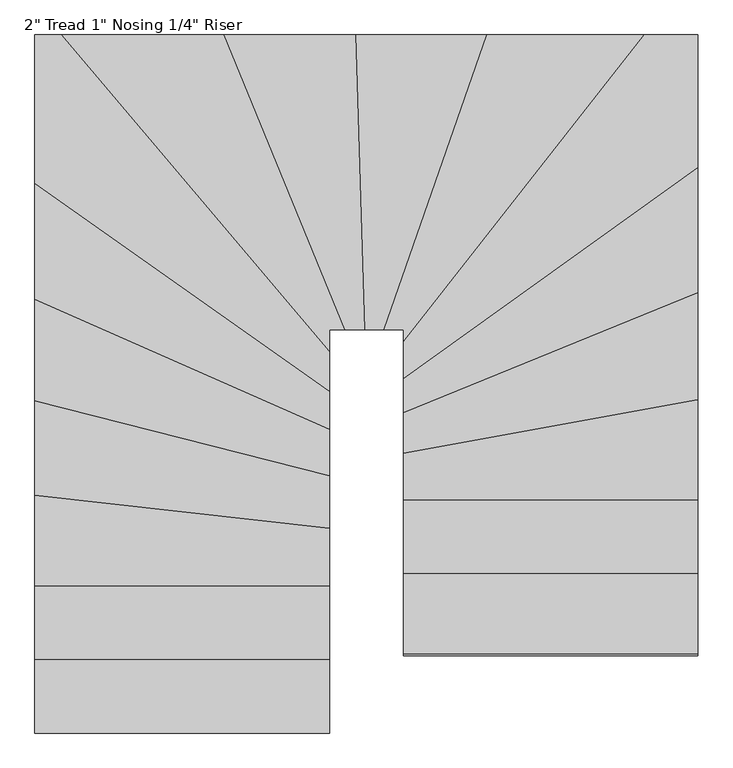
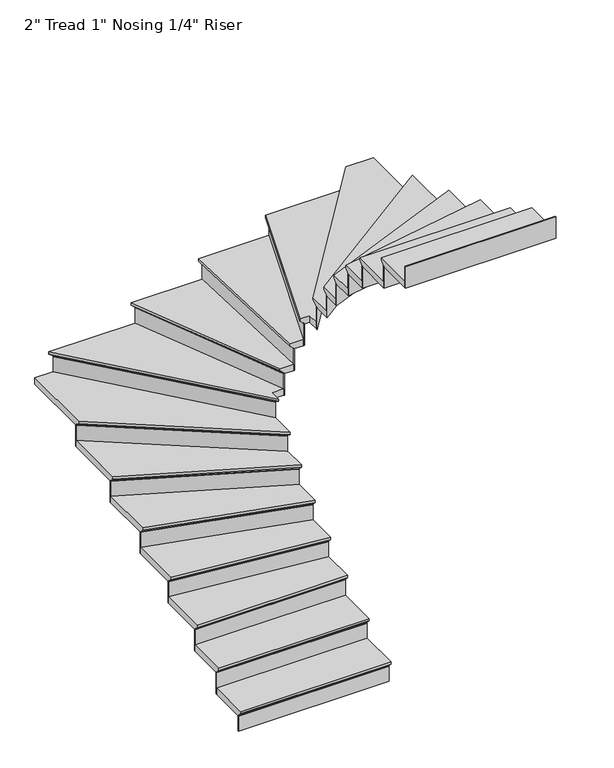
"""IFC4 building model written with IfcOpenShell, lengths in millimetres: stair flight geometry."""

from ifc_helpers import new_model, si_unit, origin, place, context, project, spatial, faceted_brep, source, transform, mapped, element, save


def stair_flight_2fadb1b5(model_context):
    return source(origin(), model_context, "Body", "Brep", [
        faceted_brep([(-7924.9808972, 1205.8606436, 150.2833333), (-7924.9808972, 1205.8606436, 169.3333333), (-9042.5808972, 1205.8606436, 169.3333333), (-9042.5808972, 1205.8606436, 150.2833333), (-7924.9808972, 1231.2606436, 124.8833333), (-9042.5808972, 1231.2606436, 124.8833333), (-7924.9808972, 1510.6606436, 169.3333333), (-9042.5808972, 1510.6606436, 169.3333333), (-9042.5808972, 1231.2606436, 118.5333333), (-9042.5808972, 1510.6606436, 118.5333333), (-7924.9808972, 1510.6606436, 118.5333333), (-7924.9808972, 1231.2606436, 118.5333333)], [[[0, 1, 2, 3]], [[4, 0, 3, 5]], [[2, 1, 6, 7]], [[8, 9, 10, 11]], [[2, 7, 9, 8, 5, 3]], [[8, 11, 4, 5]], [[6, 1, 0, 4, 11, 10]], [[7, 6, 10, 9]]]),
        faceted_brep([(-7924.9808972, 1231.2606436, 118.5333333), (-7924.9808972, 1231.2606436, 0.0), (-7924.9808972, 1237.6106436, 0.0), (-7924.9808972, 1237.6106436, 118.5333333), (-9042.5808972, 1231.2606436, 118.5333333), (-9042.5808972, 1237.6106436, 118.5333333), (-9042.5808972, 1237.6106436, 0.0), (-9042.5808972, 1231.2606436, 0.0)], [[[0, 1, 2, 3]], [[4, 5, 6, 7]], [[1, 0, 4, 7]], [[2, 1, 7, 6]], [[3, 2, 6, 5]], [[0, 3, 5, 4]]]),
        faceted_brep([(-7924.9808972, 1510.6606436, 287.8666667), (-7924.9808972, 1510.6606436, 118.5333333), (-7924.9808972, 1517.0106436, 118.5333333), (-7924.9808972, 1517.0106436, 287.8666667), (-9042.5808972, 1510.6606436, 287.8666667), (-9042.5808972, 1517.0106436, 287.8666667), (-9042.5808972, 1517.0106436, 118.5333333), (-9042.5808972, 1510.6606436, 118.5333333)], [[[0, 1, 2, 3]], [[4, 5, 6, 7]], [[1, 0, 4, 7]], [[2, 1, 7, 6]], [[3, 2, 6, 5]], [[0, 3, 5, 4]]]),
        faceted_brep([(-9042.5808972, 1485.2606436, 338.6666667), (-7924.9808972, 1485.2606436, 338.6666667), (-7924.9808972, 1790.0606436, 338.6666667), (-9042.5808972, 1790.0606436, 338.6666667), (-9042.5808972, 1510.6606436, 287.8666667), (-9042.5808972, 1790.0606436, 287.8666667), (-7924.9808972, 1790.0606436, 287.8666667), (-7924.9808972, 1510.6606436, 287.8666667), (-9042.5808972, 1510.6606436, 294.2166667), (-9042.5808972, 1485.2606436, 319.6166667), (-7924.9808972, 1510.6606436, 294.2166667), (-7924.9808972, 1485.2606436, 319.6166667)], [[[0, 1, 2, 3]], [[4, 5, 6, 7]], [[0, 3, 5, 4, 8, 9]], [[4, 7, 10, 8]], [[2, 1, 11, 10, 7, 6]], [[3, 2, 6, 5]], [[11, 1, 0, 9]], [[10, 11, 9, 8]]]),
        faceted_brep([(-7924.9808972, 1790.0606436, 457.2), (-7924.9808972, 1790.0606436, 287.8666667), (-7924.9808972, 1796.4106436, 287.8666667), (-7924.9808972, 1796.4106436, 457.2), (-9042.5808972, 1790.0606436, 457.2), (-9042.5808972, 1796.4106436, 457.2), (-9042.5808972, 1796.4106436, 287.8666667), (-9042.5808972, 1790.0606436, 287.8666667)], [[[0, 1, 2, 3]], [[4, 5, 6, 7]], [[1, 0, 4, 7]], [[2, 1, 7, 6]], [[3, 2, 6, 5]], [[0, 3, 5, 4]]]),
        faceted_brep([(-9042.5808972, 1764.6606436, 508.0), (-7924.9808972, 1764.6606436, 508.0), (-7924.9808972, 2006.9009022, 508.0), (-9042.5808972, 2132.3393631, 508.0), (-9042.5808972, 1790.0606436, 457.2), (-9042.5808972, 2132.3393631, 457.2), (-7924.9808972, 2006.9009022, 457.2), (-7924.9808972, 1790.0606436, 457.2), (-9042.5808972, 1790.0606436, 463.55), (-9042.5808972, 1764.6606436, 488.95), (-7924.9808972, 1790.0606436, 463.55), (-7924.9808972, 1764.6606436, 488.95)], [[[0, 1, 2, 3]], [[4, 5, 6, 7]], [[0, 3, 5, 4, 8, 9]], [[4, 7, 10, 8]], [[2, 1, 11, 10, 7, 6]], [[3, 2, 6, 5]], [[11, 1, 0, 9]], [[10, 11, 9, 8]]]),
        faceted_brep([(-7924.9808972, 2006.9009022, 626.5333333), (-7924.9808972, 2006.9009022, 457.2), (-7924.9808972, 2013.2907745, 457.2), (-7924.9808972, 2013.2907745, 626.5333333), (-9042.5808972, 2132.3393631, 626.5333333), (-9042.5808972, 2138.7292354, 626.5333333), (-9042.5808972, 2138.7292354, 457.2), (-9042.5808972, 2132.3393631, 457.2)], [[[0, 1, 2, 3]], [[4, 5, 6, 7]], [[1, 0, 4, 7]], [[2, 1, 7, 6]], [[3, 2, 6, 5]], [[0, 3, 5, 4]]]),
        faceted_brep([(-9042.5808972, 2106.779874, 677.3333333), (-7924.9808972, 1981.3414131, 677.3333333), (-7924.9808972, 2207.3909228, 677.3333333), (-9042.5808972, 2491.9511882, 677.3333333), (-9042.5808972, 2132.3393631, 626.5333333), (-9042.5808972, 2491.9511882, 626.5333333), (-7924.9808972, 2207.3909228, 626.5333333), (-7924.9808972, 2006.9009022, 626.5333333), (-9042.5808972, 2132.3393631, 632.8833333), (-9042.5808972, 2106.779874, 658.2833333), (-7924.9808972, 2006.9009022, 632.8833333), (-7924.9808972, 1981.3414131, 658.2833333)], [[[0, 1, 2, 3]], [[4, 5, 6, 7]], [[0, 3, 5, 4, 8, 9]], [[4, 7, 10, 8]], [[2, 1, 11, 10, 7, 6]], [[3, 2, 6, 5]], [[11, 1, 0, 9]], [[10, 11, 9, 8]]]),
        faceted_brep([(-7924.9808972, 2207.3909228, 795.8666667), (-7924.9808972, 2207.3909228, 626.5333333), (-7924.9808972, 2213.9435258, 626.5333333), (-7924.9808972, 2213.9435258, 795.8666667), (-9042.5808972, 2491.9511882, 795.8666667), (-9042.5808972, 2498.5037912, 795.8666667), (-9042.5808972, 2498.5037912, 626.5333333), (-9042.5808972, 2491.9511882, 626.5333333)], [[[0, 1, 2, 3]], [[4, 5, 6, 7]], [[1, 0, 4, 7]], [[2, 1, 7, 6]], [[3, 2, 6, 5]], [[0, 3, 5, 4]]]),
        faceted_brep([(-9042.5808972, 2465.7407763, 846.6666667), (-7924.9808972, 2181.1805109, 846.6666667), (-7924.9808972, 2384.1041471, 846.6666667), (-9042.5808972, 2877.1408478, 846.6666667), (-9042.5808972, 2491.9511882, 795.8666667), (-9042.5808972, 2877.1408478, 795.8666667), (-7924.9808972, 2384.1041471, 795.8666667), (-7924.9808972, 2207.3909228, 795.8666667), (-9042.5808972, 2491.9511882, 802.2166667), (-9042.5808972, 2465.7407763, 827.6166667), (-7924.9808972, 2207.3909228, 802.2166667), (-7924.9808972, 2181.1805109, 827.6166667)], [[[0, 1, 2, 3]], [[4, 5, 6, 7]], [[0, 3, 5, 4, 8, 9]], [[4, 7, 10, 8]], [[2, 1, 11, 10, 7, 6]], [[3, 2, 6, 5]], [[11, 1, 0, 9]], [[10, 11, 9, 8]]]),
        faceted_brep([(-7924.9808972, 2384.1041471, 965.2), (-7924.9808972, 2384.1041471, 795.8666667), (-7924.9808972, 2391.0446106, 795.8666667), (-7924.9808972, 2391.0446106, 965.2), (-9042.5808972, 2877.1408478, 965.2), (-9042.5808972, 2884.0813113, 965.2), (-9042.5808972, 2884.0813113, 795.8666667), (-9042.5808972, 2877.1408478, 795.8666667)], [[[0, 1, 2, 3]], [[4, 5, 6, 7]], [[1, 0, 4, 7]], [[2, 1, 7, 6]], [[3, 2, 6, 5]], [[0, 3, 5, 4]]]),
        faceted_brep([(-9042.5808972, 2849.3789939, 1016.0), (-7924.9808972, 2356.3422932, 1016.0), (-7924.9808972, 2533.0028357, 1016.0), (-9042.5808972, 3320.3326574, 1016.0), (-9042.5808972, 2877.1408478, 965.2), (-9042.5808972, 3320.3326574, 965.2), (-7924.9808972, 2533.0028357, 965.2), (-7924.9808972, 2384.1041471, 965.2), (-9042.5808972, 2877.1408478, 971.55), (-9042.5808972, 2849.3789939, 996.95), (-7924.9808972, 2384.1041471, 971.55), (-7924.9808972, 2356.3422932, 996.95)], [[[0, 1, 2, 3]], [[4, 5, 6, 7]], [[0, 3, 5, 4, 8, 9]], [[4, 7, 10, 8]], [[2, 1, 11, 10, 7, 6]], [[3, 2, 6, 5]], [[11, 1, 0, 9]], [[10, 11, 9, 8]]]),
        faceted_brep([(-7924.9808972, 2533.0028357, 1134.5333333), (-7924.9808972, 2533.0028357, 965.2), (-7924.9808972, 2540.770357, 965.2), (-7924.9808972, 2540.770357, 1134.5333333), (-9042.5808972, 3320.3326574, 1134.5333333), (-9042.5808972, 3328.1001788, 1134.5333333), (-9042.5808972, 3328.1001788, 965.2), (-9042.5808972, 3320.3326574, 965.2)], [[[0, 1, 2, 3]], [[4, 5, 6, 7]], [[1, 0, 4, 7]], [[2, 1, 7, 6]], [[3, 2, 6, 5]], [[0, 3, 5, 4]]]),
        faceted_brep([(-8907.7976269, 3851.1923354, 1185.3333333), (-9042.5808972, 3851.1923354, 1185.3333333), (-9042.5808972, 3289.2625719, 1185.3333333), (-7924.9808972, 2501.9327502, 1185.3333333), (-7924.9808972, 2691.3009895, 1185.3333333), (-9042.5808972, 3851.1923354, 1134.5333333), (-8907.7976269, 3851.1923354, 1134.5333333), (-7924.9808972, 2691.3009895, 1134.5333333), (-7924.9808972, 2533.0028357, 1134.5333333), (-9042.5808972, 3320.3326574, 1134.5333333), (-9042.5808972, 3320.3326574, 1140.8833333), (-9042.5808972, 3289.2625719, 1166.2833333), (-7924.9808972, 2533.0028357, 1140.8833333), (-7924.9808972, 2501.9327502, 1166.2833333)], [[[0, 1, 2, 3, 4]], [[5, 6, 7, 8, 9]], [[1, 0, 6, 5]], [[2, 1, 5, 9, 10, 11]], [[9, 8, 12, 10]], [[4, 3, 13, 12, 8, 7]], [[0, 4, 7, 6]], [[13, 3, 2, 11]], [[12, 13, 11, 10]]]),
        faceted_brep([(-7924.9808972, 2691.3009895, 1303.8666667), (-7924.9808972, 2691.3009895, 1134.5333333), (-7924.9808972, 2701.1236052, 1134.5333333), (-7924.9808972, 2701.1236052, 1303.8666667), (-8907.7976269, 3851.1923354, 1303.8666667), (-8899.4745792, 3851.1923354, 1303.8666667), (-8899.4745792, 3851.1923354, 1134.5333333), (-8907.7976269, 3851.1923354, 1134.5333333)], [[[0, 1, 2, 3]], [[4, 5, 6, 7]], [[1, 0, 4, 7]], [[2, 1, 7, 6]], [[3, 2, 6, 5]], [[0, 3, 5, 4]]]),
        faceted_brep([(-8941.0898177, 3851.1923354, 1354.6666667), (-7924.9808972, 2652.0105269, 1354.6666667), (-7924.9808972, 2733.5923354, 1354.6666667), (-7838.5095187, 2733.5923354, 1354.6666667), (-8297.8208023, 3851.1923354, 1354.6666667), (-8907.7976269, 3851.1923354, 1303.8666667), (-8297.8208023, 3851.1923354, 1303.8666667), (-7838.5095187, 2733.5923354, 1303.8666667), (-7924.9808972, 2733.5923354, 1303.8666667), (-7924.9808972, 2691.3009895, 1303.8666667), (-8907.7976269, 3851.1923354, 1310.2166667), (-8941.0898177, 3851.1923354, 1335.6166667), (-7924.9808972, 2691.3009895, 1310.2166667), (-7924.9808972, 2652.0105269, 1335.6166667)], [[[0, 1, 2, 3, 4]], [[5, 6, 7, 8, 9]], [[0, 4, 6, 5, 10, 11]], [[5, 9, 12, 10]], [[3, 2, 8, 7]], [[4, 3, 7, 6]], [[13, 1, 0, 11]], [[12, 13, 11, 10]], [[2, 1, 13, 12, 9, 8]]]),
        faceted_brep([(-7838.5095187, 2733.5923354, 1473.2), (-7838.5095187, 2733.5923354, 1303.8666667), (-7831.6441596, 2733.5923354, 1303.8666667), (-7831.6441596, 2733.5923354, 1473.2), (-8297.8208023, 3851.1923354, 1473.2), (-8290.9554433, 3851.1923354, 1473.2), (-8290.9554433, 3851.1923354, 1303.8666667), (-8297.8208023, 3851.1923354, 1303.8666667)], [[[0, 1, 2, 3]], [[4, 5, 6, 7]], [[1, 0, 4, 7]], [[2, 1, 7, 6]], [[3, 2, 6, 5]], [[0, 3, 5, 4]]]),
        faceted_brep([(-8325.2822386, 3851.1923354, 1524.0), (-7865.970955, 2733.5923354, 1524.0), (-7765.6019906, 2733.5923354, 1524.0), (-7798.581504, 3851.1923354, 1524.0), (-8297.8208023, 3851.1923354, 1473.2), (-7798.581504, 3851.1923354, 1473.2), (-7765.6019906, 2733.5923354, 1473.2), (-7838.5095187, 2733.5923354, 1473.2), (-8297.8208023, 3851.1923354, 1479.55), (-8325.2822386, 3851.1923354, 1504.95), (-7838.5095187, 2733.5923354, 1479.55), (-7865.970955, 2733.5923354, 1504.95)], [[[0, 1, 2, 3]], [[4, 5, 6, 7]], [[0, 3, 5, 4, 8, 9]], [[4, 7, 10, 8]], [[2, 1, 11, 10, 7, 6]], [[3, 2, 6, 5]], [[11, 1, 0, 9]], [[10, 11, 9, 8]]]),
        faceted_brep([(-7765.6019906, 2733.5923354, 1642.5333333), (-7765.6019906, 2733.5923354, 1473.2), (-7759.2492264, 2733.5923354, 1473.2), (-7759.2492264, 2733.5923354, 1642.5333333), (-7798.581504, 3851.1923354, 1642.5333333), (-7792.2287398, 3851.1923354, 1642.5333333), (-7792.2287398, 3851.1923354, 1473.2), (-7798.581504, 3851.1923354, 1473.2)], [[[0, 1, 2, 3]], [[4, 5, 6, 7]], [[1, 0, 4, 7]], [[2, 1, 7, 6]], [[3, 2, 6, 5]], [[0, 3, 5, 4]]]),
        faceted_brep([(-7823.9925607, 3851.1923354, 1693.3333333), (-7791.0130473, 2733.5923354, 1693.3333333), (-7692.111373, 2733.5923354, 1693.3333333), (-7302.1708713, 3851.1923354, 1693.3333333), (-7798.581504, 3851.1923354, 1642.5333333), (-7302.1708713, 3851.1923354, 1642.5333333), (-7692.111373, 2733.5923354, 1642.5333333), (-7765.6019906, 2733.5923354, 1642.5333333), (-7798.581504, 3851.1923354, 1648.8833333), (-7823.9925607, 3851.1923354, 1674.2833333), (-7765.6019906, 2733.5923354, 1648.8833333), (-7791.0130473, 2733.5923354, 1674.2833333)], [[[0, 1, 2, 3]], [[4, 5, 6, 7]], [[0, 3, 5, 4, 8, 9]], [[4, 7, 10, 8]], [[2, 1, 11, 10, 7, 6]], [[3, 2, 6, 5]], [[11, 1, 0, 9]], [[10, 11, 9, 8]]]),
        faceted_brep([(-7692.111373, 2733.5923354, 1811.8666667), (-7692.111373, 2733.5923354, 1642.5333333), (-7685.3859544, 2733.5923354, 1642.5333333), (-7685.3859544, 2733.5923354, 1811.8666667), (-7302.1708713, 3851.1923354, 1811.8666667), (-7295.4454527, 3851.1923354, 1811.8666667), (-7295.4454527, 3851.1923354, 1642.5333333), (-7302.1708713, 3851.1923354, 1642.5333333)], [[[0, 1, 2, 3]], [[4, 5, 6, 7]], [[1, 0, 4, 7]], [[2, 1, 7, 6]], [[3, 2, 6, 5]], [[0, 3, 5, 4]]]),
        faceted_brep([(-7329.0725456, 3851.1923354, 1862.6666667), (-7719.0130473, 2733.5923354, 1862.6666667), (-7645.5808972, 2733.5923354, 1862.6666667), (-7645.5808972, 2646.5119616, 1862.6666667), (-6699.3018022, 3851.1923354, 1862.6666667), (-7302.1708713, 3851.1923354, 1811.8666667), (-6699.3018022, 3851.1923354, 1811.8666667), (-7645.5808972, 2646.5119616, 1811.8666667), (-7645.5808972, 2733.5923354, 1811.8666667), (-7692.111373, 2733.5923354, 1811.8666667), (-7302.1708713, 3851.1923354, 1818.2166667), (-7329.0725456, 3851.1923354, 1843.6166667), (-7692.111373, 2733.5923354, 1818.2166667), (-7719.0130473, 2733.5923354, 1843.6166667)], [[[0, 1, 2, 3, 4]], [[5, 6, 7, 8, 9]], [[0, 4, 6, 5, 10, 11]], [[5, 9, 12, 10]], [[2, 1, 13, 12, 9, 8]], [[4, 3, 7, 6]], [[13, 1, 0, 11]], [[12, 13, 11, 10]], [[3, 2, 8, 7]]]),
        faceted_brep([(-7645.5808972, 2646.5119616, 1981.2), (-7645.5808972, 2646.5119616, 1811.8666667), (-7645.5808972, 2636.2321971, 1811.8666667), (-7645.5808972, 2636.2321971, 1981.2), (-6699.3018022, 3851.1923354, 1981.2), (-6691.2270245, 3851.1923354, 1981.2), (-6691.2270245, 3851.1923354, 1811.8666667), (-6699.3018022, 3851.1923354, 1811.8666667)], [[[0, 1, 2, 3]], [[4, 5, 6, 7]], [[1, 0, 4, 7]], [[2, 1, 7, 6]], [[3, 2, 6, 5]], [[0, 3, 5, 4]]]),
        faceted_brep([(-6527.9808972, 3317.4403684, 2032.0), (-6527.9808972, 3851.1923354, 2032.0), (-6731.6009132, 3851.1923354, 2032.0), (-7645.5808972, 2687.6310198, 2032.0), (-7645.5808972, 2517.3671111, 2032.0), (-6527.9808972, 3851.1923354, 1981.2), (-6527.9808972, 3317.4403684, 1981.2), (-7645.5808972, 2517.3671111, 1981.2), (-7645.5808972, 2646.5119616, 1981.2), (-6699.3018022, 3851.1923354, 1981.2), (-7645.5808972, 2646.5119616, 1987.55), (-6699.3018022, 3851.1923354, 1987.55), (-7645.5808972, 2687.6310198, 2012.95), (-6731.6009132, 3851.1923354, 2012.95)], [[[0, 1, 2, 3, 4]], [[5, 6, 7, 8, 9]], [[1, 0, 6, 5]], [[9, 8, 10, 11]], [[4, 3, 12, 10, 8, 7]], [[0, 4, 7, 6]], [[12, 3, 2, 13]], [[10, 12, 13, 11]], [[2, 1, 5, 9, 11, 13]]]),
        faceted_brep([(-7645.5808972, 2517.3671111, 2150.5333333), (-7645.5808972, 2517.3671111, 1981.2), (-7645.5808972, 2509.5576655, 1981.2), (-7645.5808972, 2509.5576655, 2150.5333333), (-6527.9808972, 3317.4403684, 2150.5333333), (-6527.9808972, 3309.6309228, 2150.5333333), (-6527.9808972, 3309.6309228, 1981.2), (-6527.9808972, 3317.4403684, 1981.2)], [[[0, 1, 2, 3]], [[4, 5, 6, 7]], [[1, 0, 4, 7]], [[2, 1, 7, 6]], [[3, 2, 6, 5]], [[0, 3, 5, 4]]]),
        faceted_brep([(-6527.9808972, 3348.678151, 2201.3333333), (-7645.5808972, 2548.6048936, 2201.3333333), (-7645.5808972, 2392.4773927, 2201.3333333), (-6527.9808972, 2847.0609144, 2201.3333333), (-6527.9808972, 3317.4403684, 2150.5333333), (-6527.9808972, 2847.0609144, 2150.5333333), (-7645.5808972, 2392.4773927, 2150.5333333), (-7645.5808972, 2517.3671111, 2150.5333333), (-6527.9808972, 3317.4403684, 2156.8833333), (-6527.9808972, 3348.678151, 2182.2833333), (-7645.5808972, 2517.3671111, 2156.8833333), (-7645.5808972, 2548.6048936, 2182.2833333)], [[[0, 1, 2, 3]], [[4, 5, 6, 7]], [[0, 3, 5, 4, 8, 9]], [[4, 7, 10, 8]], [[2, 1, 11, 10, 7, 6]], [[3, 2, 6, 5]], [[11, 1, 0, 9]], [[10, 11, 9, 8]]]),
        faceted_brep([(-7645.5808972, 2392.4773927, 2319.8666667), (-7645.5808972, 2392.4773927, 2150.5333333), (-7645.5808972, 2385.6221998, 2150.5333333), (-7645.5808972, 2385.6221998, 2319.8666667), (-6527.9808972, 2847.0609144, 2319.8666667), (-6527.9808972, 2840.2057215, 2319.8666667), (-6527.9808972, 2840.2057215, 2150.5333333), (-6527.9808972, 2847.0609144, 2150.5333333)], [[[0, 1, 2, 3]], [[4, 5, 6, 7]], [[1, 0, 4, 7]], [[2, 1, 7, 6]], [[3, 2, 6, 5]], [[0, 3, 5, 4]]]),
        faceted_brep([(-6527.9808972, 2874.4816863, 2370.6666667), (-7645.5808972, 2419.8981646, 2370.6666667), (-7645.5808972, 2240.9879192, 2370.6666667), (-6527.9808972, 2442.9689719, 2370.6666667), (-6527.9808972, 2847.0609144, 2319.8666667), (-6527.9808972, 2442.9689719, 2319.8666667), (-7645.5808972, 2240.9879192, 2319.8666667), (-7645.5808972, 2392.4773927, 2319.8666667), (-6527.9808972, 2847.0609144, 2326.2166667), (-6527.9808972, 2874.4816863, 2351.6166667), (-7645.5808972, 2392.4773927, 2326.2166667), (-7645.5808972, 2419.8981646, 2351.6166667)], [[[0, 1, 2, 3]], [[4, 5, 6, 7]], [[0, 3, 5, 4, 8, 9]], [[4, 7, 10, 8]], [[2, 1, 11, 10, 7, 6]], [[3, 2, 6, 5]], [[11, 1, 0, 9]], [[10, 11, 9, 8]]]),
        faceted_brep([(-7645.5808972, 2240.9879192, 2489.2), (-7645.5808972, 2240.9879192, 2319.8666667), (-7645.5808972, 2234.5350493, 2319.8666667), (-7645.5808972, 2234.5350493, 2489.2), (-6527.9808972, 2442.9689719, 2489.2), (-6527.9808972, 2436.5161019, 2489.2), (-6527.9808972, 2436.5161019, 2319.8666667), (-6527.9808972, 2442.9689719, 2319.8666667)], [[[0, 1, 2, 3]], [[4, 5, 6, 7]], [[1, 0, 4, 7]], [[2, 1, 7, 6]], [[3, 2, 6, 5]], [[0, 3, 5, 4]]]),
        faceted_brep([(-6527.9808972, 2468.7804518, 2540.0), (-7645.5808972, 2266.7993991, 2540.0), (-7645.5808972, 2062.9899254, 2540.0), (-6527.9808972, 2062.9899254, 2540.0), (-6527.9808972, 2442.9689719, 2489.2), (-6527.9808972, 2062.9899254, 2489.2), (-7645.5808972, 2062.9899254, 2489.2), (-7645.5808972, 2240.9879192, 2489.2), (-6527.9808972, 2442.9689719, 2495.55), (-6527.9808972, 2468.7804518, 2520.95), (-7645.5808972, 2240.9879192, 2495.55), (-7645.5808972, 2266.7993991, 2520.95)], [[[0, 1, 2, 3]], [[4, 5, 6, 7]], [[0, 3, 5, 4, 8, 9]], [[4, 7, 10, 8]], [[2, 1, 11, 10, 7, 6]], [[3, 2, 6, 5]], [[11, 1, 0, 9]], [[10, 11, 9, 8]]]),
        faceted_brep([(-7645.5808972, 2062.9899254, 2658.5333333), (-7645.5808972, 2062.9899254, 2489.2), (-7645.5808972, 2056.6399254, 2489.2), (-7645.5808972, 2056.6399254, 2658.5333333), (-6527.9808972, 2062.9899254, 2658.5333333), (-6527.9808972, 2056.6399254, 2658.5333333), (-6527.9808972, 2056.6399254, 2489.2), (-6527.9808972, 2062.9899254, 2489.2)], [[[0, 1, 2, 3]], [[4, 5, 6, 7]], [[1, 0, 4, 7]], [[2, 1, 7, 6]], [[3, 2, 6, 5]], [[0, 3, 5, 4]]]),
        faceted_brep([(-6527.9808972, 2088.3899254, 2709.3333333), (-7645.5808972, 2088.3899254, 2709.3333333), (-7645.5808972, 1783.5899254, 2709.3333333), (-6527.9808972, 1783.5899254, 2709.3333333), (-6527.9808972, 2062.9899254, 2658.5333333), (-6527.9808972, 1783.5899254, 2658.5333333), (-7645.5808972, 1783.5899254, 2658.5333333), (-7645.5808972, 2062.9899254, 2658.5333333), (-6527.9808972, 2062.9899254, 2664.8833333), (-6527.9808972, 2088.3899254, 2690.2833333), (-7645.5808972, 2062.9899254, 2664.8833333), (-7645.5808972, 2088.3899254, 2690.2833333)], [[[0, 1, 2, 3]], [[4, 5, 6, 7]], [[0, 3, 5, 4, 8, 9]], [[4, 7, 10, 8]], [[2, 1, 11, 10, 7, 6]], [[3, 2, 6, 5]], [[11, 1, 0, 9]], [[10, 11, 9, 8]]]),
        faceted_brep([(-7645.5808972, 1783.5899254, 2827.8666667), (-7645.5808972, 1783.5899254, 2658.5333333), (-7645.5808972, 1777.2399254, 2658.5333333), (-7645.5808972, 1777.2399254, 2827.8666667), (-6527.9808972, 1783.5899254, 2827.8666667), (-6527.9808972, 1777.2399254, 2827.8666667), (-6527.9808972, 1777.2399254, 2658.5333333), (-6527.9808972, 1783.5899254, 2658.5333333)], [[[0, 1, 2, 3]], [[4, 5, 6, 7]], [[1, 0, 4, 7]], [[2, 1, 7, 6]], [[3, 2, 6, 5]], [[0, 3, 5, 4]]]),
        faceted_brep([(-7645.5808972, 1504.1899254, 2997.2), (-7645.5808972, 1504.1899254, 2827.8666667), (-7645.5808972, 1497.8399254, 2827.8666667), (-7645.5808972, 1497.8399254, 2997.2), (-6527.9808972, 1504.1899254, 2997.2), (-6527.9808972, 1497.8399254, 2997.2), (-6527.9808972, 1497.8399254, 2827.8666667), (-6527.9808972, 1504.1899254, 2827.8666667)], [[[0, 1, 2, 3]], [[4, 5, 6, 7]], [[1, 0, 4, 7]], [[2, 1, 7, 6]], [[3, 2, 6, 5]], [[0, 3, 5, 4]]]),
        faceted_brep([(-6527.9808972, 1808.9899254, 2878.6666667), (-7645.5808972, 1808.9899254, 2878.6666667), (-7645.5808972, 1504.1899254, 2878.6666667), (-6527.9808972, 1504.1899254, 2878.6666667), (-6527.9808972, 1783.5899254, 2827.8666667), (-6527.9808972, 1504.1899254, 2827.8666667), (-7645.5808972, 1504.1899254, 2827.8666667), (-7645.5808972, 1783.5899254, 2827.8666667), (-6527.9808972, 1783.5899254, 2834.2166667), (-6527.9808972, 1808.9899254, 2859.6166667), (-7645.5808972, 1783.5899254, 2834.2166667), (-7645.5808972, 1808.9899254, 2859.6166667)], [[[0, 1, 2, 3]], [[4, 5, 6, 7]], [[0, 3, 5, 4, 8, 9]], [[4, 7, 10, 8]], [[2, 1, 11, 10, 7, 6]], [[3, 2, 6, 5]], [[11, 1, 0, 9]], [[10, 11, 9, 8]]]),
    ])


if __name__ == "__main__":
    model = new_model("IFC4")
    model_context = context("Model", 3, world=origin())
    ifc_project = project(units=[si_unit("LENGTHUNIT", "METRE", prefix="MILLI")], contexts=[model_context])
    site = spatial("IfcSite", under=ifc_project)
    building = spatial("IfcBuilding", under=site)
    placement = place(None, origin())
    stair_flight_shape = stair_flight_2fadb1b5(model_context)
    element("IfcStairFlight", 1, ObjectType="2\" Tread 1\" Nosing 1/4\" Riser", at=placement, inside=building, context=model_context, shape_type="MappedRepresentation", body=[
        mapped(stair_flight_shape, transform((0.0, 0.0, 0.0), x_axis=(1.0, 0.0, 0.0), y_axis=(0.0, 1.0, 0.0), z_axis=(0.0, 0.0, 1.0))),
    ])
    save(model, "model.ifc")
